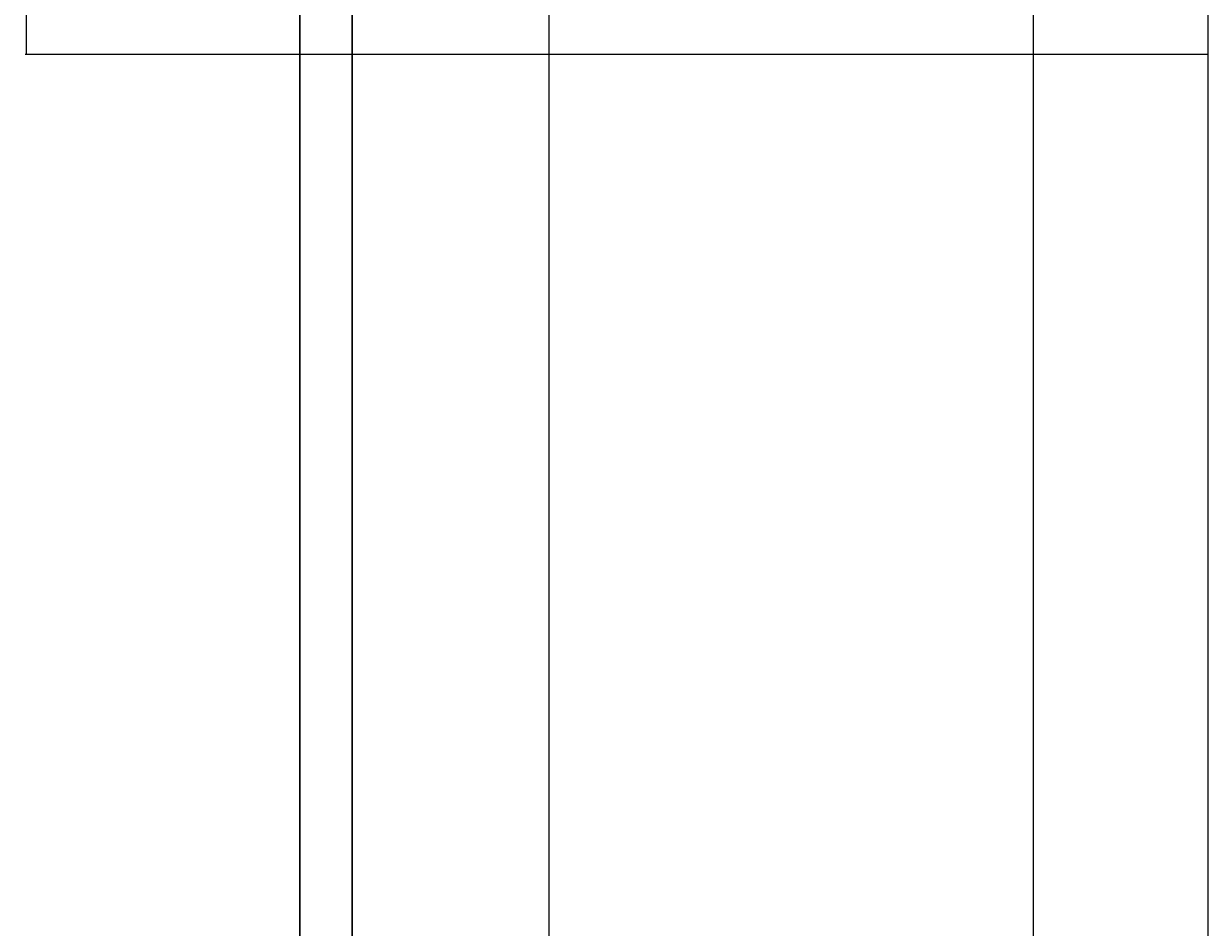
# Model space of a CAD drawing. Units: inches. Extents: x 867 to 1667, y -234 to 788.
# Tile 27 of 42: x 867 to 1071, y 417 to 572. Entities that reach past the tile are written whole.
import ezdxf

# ---------------------------------------------------------------- set-up
doc = ezdxf.new("R2010")
doc.units = ezdxf.units.IN
doc.header["$MEASUREMENT"] = 0
doc.layers.add('A-ANNO-DIMS', color=2, linetype='Continuous', lineweight=18)
doc.layers.add('A-WALL-SITE', color=8, linetype='Continuous', lineweight=30)
doc.styles.get("Standard").update_dxf_attribs({"font": 'arial.ttf'})
doc.dimstyles.get("Standard").update_dxf_attribs({"dimtxt": 0.6875, "dimasz": 0.18, "dimexe": 0.18, "dimexo": 0.0625, "dimgap": 0.09, "dimtad": 0, "dimdec": 4, "dimzin": 0, "dimdsep": 46, "dimlunit": 4, "dimtxsty": 'Standard', "dimcen": 0.09, "dimadec": 0, "dimazin": 0, "dimtfac": 1, "dimtdec": 4, "dimtofl": 0, "dimtmove": 0, "dimatfit": 3, "dimfxl": 1, "dimtolj": 1, "dimtzin": 0, "dimarcsym": 0})

# ---------------------------------------------------------------- blocks, each defined once
blk = doc.blocks.new('*D24')
at = {"layer": 'A-ANNO-DIMS', "color": 0, "lineweight": -2, "transparency": 16777216}
for p, q in [((1067.82, 623.62), (867.76, 623.62)), ((867.94, 623.44), (867.94, 595.7)), ((867.94, 566.8), (867.94, 594.53)), ((1070.82, 566.62), (867.76, 566.62))]:
    blk.add_line(p, q, dxfattribs=at)
at = {"layer": 'A-ANNO-DIMS', "color": 0, "transparency": 16777216}
for points in [[(867.91, 623.44), (867.97, 623.44), (867.94, 623.62)], [(867.91, 566.8), (867.97, 566.8), (867.94, 566.62)]]:
    blk.add_solid(points, dxfattribs=at)
at = {"layer": 'Defpoints', "color": 0, "transparency": 16777216}
for p in [(1067.89, 623.62), (867.94, 566.62), (1070.89, 566.62)]:
    blk.add_point(p, dxfattribs=at)
at = {"layer": 'A-ANNO-DIMS', "color": 0, "transparency": 16777216, "insert": (867.94, 595.12), "char_height": 0.688, "attachment_point": 5, "rotation": 90}
blk.add_mtext('\\A1;57', dxfattribs=at)
blk = doc.blocks.new('*D28')
at = {"layer": 'A-ANNO-DIMS', "color": 0, "lineweight": -2, "transparency": 16777216}
for p, q in [((914.89, 623.55), (914.89, -233.54)), ((957.64, 623.55), (957.64, -233.54)), ((915.07, -233.36), (935, -233.36)), ((957.46, -233.36), (937.53, -233.36))]:
    blk.add_line(p, q, dxfattribs=at)
at = {"layer": 'A-ANNO-DIMS', "color": 0, "transparency": 16777216}
for points in [[(915.07, -233.33), (915.07, -233.39), (914.89, -233.36)], [(957.46, -233.33), (957.46, -233.39), (957.64, -233.36)]]:
    blk.add_solid(points, dxfattribs=at)
at = {"layer": 'Defpoints', "color": 0, "transparency": 16777216}
for p in [(914.89, 623.62), (957.64, 623.62), (914.89, -233.36)]:
    blk.add_point(p, dxfattribs=at)
at = {"layer": 'A-ANNO-DIMS', "color": 0, "transparency": 16777216, "insert": (936.26, -233.36), "char_height": 0.688, "attachment_point": 5}
blk.add_mtext('\\A1;42.75', dxfattribs=at)
blk = doc.blocks.new('*D31')
at = {"layer": 'A-ANNO-DIMS', "color": 0, "lineweight": -2, "transparency": 16777216}
for p, q in [((1070.89, 566.68), (1070.89, 787.75)), ((1071.07, 787.57), (1304.02, 787.57)), ((1538.71, 787.57), (1305.75, 787.57)), ((1538.89, 566.68), (1538.89, 787.75))]:
    blk.add_line(p, q, dxfattribs=at)
at = {"layer": 'A-ANNO-DIMS', "color": 0, "transparency": 16777216}
for points in [[(1071.07, 787.6), (1071.07, 787.54), (1070.89, 787.57)], [(1538.71, 787.6), (1538.71, 787.54), (1538.89, 787.57)]]:
    blk.add_solid(points, dxfattribs=at)
at = {"layer": 'Defpoints', "color": 0, "transparency": 16777216}
for p in [(1538.89, 787.57), (1070.89, 566.62), (1538.89, 566.62)]:
    blk.add_point(p, dxfattribs=at)
at = {"layer": 'A-ANNO-DIMS', "color": 0, "transparency": 16777216, "insert": (1304.89, 787.57), "char_height": 0.688, "attachment_point": 5}
blk.add_mtext('\\A1;468', dxfattribs=at)
blk = doc.blocks.new('*D35')
at = {"layer": 'A-ANNO-DIMS', "color": 0, "lineweight": -2, "transparency": 16777216}
for p, q in [((1040.89, 413.68), (1040.89, 787.75)), ((1041.07, 787.57), (1055.31, 787.57)), ((1070.71, 787.57), (1056.47, 787.57)), ((1070.89, 404.68), (1070.89, 787.75))]:
    blk.add_line(p, q, dxfattribs=at)
at = {"layer": 'A-ANNO-DIMS', "color": 0, "transparency": 16777216}
for points in [[(1041.07, 787.6), (1041.07, 787.54), (1040.89, 787.57)], [(1070.71, 787.6), (1070.71, 787.54), (1070.89, 787.57)]]:
    blk.add_solid(points, dxfattribs=at)
at = {"layer": 'Defpoints', "color": 0, "transparency": 16777216}
for p in [(1070.89, 787.57), (1040.89, 413.62), (1070.89, 404.62)]:
    blk.add_point(p, dxfattribs=at)
at = {"layer": 'A-ANNO-DIMS', "color": 0, "transparency": 16777216, "insert": (1055.89, 787.57), "char_height": 0.688, "attachment_point": 5}
blk.add_mtext('\\A1;30', dxfattribs=at)

msp = doc.modelspace()

# ---------------------------------------------------------------- linework, layer by layer
at = {"layer": 'A-WALL-SITE'}
for p, q in [((914.8866, 740.617), (914.8866, -186.4081)), ((923.8866, 740.617), (923.8866, -186.4081))]:
    msp.add_line(p, q, dxfattribs=at)

# ---------------------------------------------------------------- dimensions: what is measured, and where the dimension line sits
at = {"layer": 'A-ANNO-DIMS'}
for base, p1, p2, override, picture, middle in [((1070.8866, 787.567), (1040.8866, 413.617), (1070.8866, 404.617), {"dimdec": 0, "dimlfac": 1, "dimrnd": 0, "dimzin": 0, "dimdsep": 46, "dimlunit": 2}, '*D35', (1055.8866, 787.567)), ((1538.8866, 787.567), (1070.8866, 566.617), (1538.8866, 566.617), {"dimdec": 0, "dimlfac": 1, "dimrnd": 0, "dimzin": 0, "dimdsep": 46, "dimlunit": 2}, '*D31', (1304.8866, 787.567)), ((914.8866, -233.3581), (957.6375, 623.617), (914.8866, 623.617), {"dimdec": 2, "dimlfac": 1, "dimrnd": 0, "dimzin": 0, "dimdsep": 46, "dimlunit": 2}, '*D28', (936.2621, -233.3581))]:
    dim = msp.add_linear_dim(base=base, p1=p1, p2=p2, dimstyle='Standard', override=override, dxfattribs=at)
    dim.commit()
    dim.dimension.update_dxf_attribs({"geometry": picture, "text_midpoint": middle})
dim = msp.add_linear_dim(base=(867.9366, 566.617), p1=(1067.8866, 623.617), p2=(1070.8866, 566.617), angle=90, dimstyle='Standard', override={"dimdec": 0, "dimlfac": 1, "dimrnd": 0, "dimzin": 0, "dimdsep": 46, "dimlunit": 2}, dxfattribs=at)
dim.commit()
dim.dimension.update_dxf_attribs({"geometry": '*D24', "text_midpoint": (867.9366, 595.117)})

doc.saveas('drawing.dxf')
